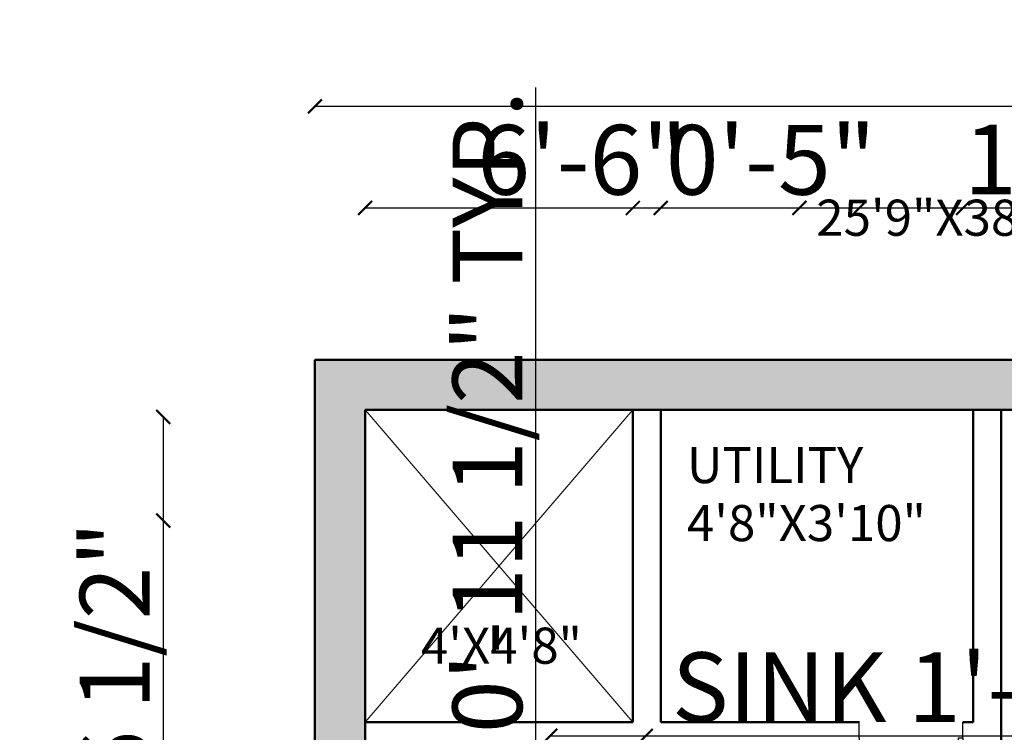
# Model space of a CAD drawing. Units: inches. Extents: x 2419 to 2878, y 1068 to 1713.
# Tile 15 of 20: x 2419 to 2595, y 1511 to 1639. Entities that reach past the tile are written whole.
import ezdxf

# ---------------------------------------------------------------- set-up
doc = ezdxf.new("R2010")
doc.units = ezdxf.units.IN
for name, color, linetype, lineweight in [('A-ANNO-DIMS', 2, 'Continuous', 18), ('A-ANNO-TEXT', 7, 'Continuous', 25), ('A-AREA-IDEN', 7, 'Continuous', 18), ('A-DOOR', 4, 'Continuous', 25), ('A-FLOR-OTLN', 8, 'Continuous', 13), ('A-FLOR-PRKG-PATT', 1, 'Continuous', 13), ('A-FURN-PATT', 254, 'Continuous', 13), ('A-WALL', 7, 'Continuous', 50)]:
    doc.layers.add(name, color=color, linetype=linetype, lineweight=lineweight)
doc.layers.add('A-FLOR-FIXT-PATT', color=254, linetype='Continuous', lineweight=13, true_color=0xd7ebd2)
doc.layers.add('A-WALL-PATT', color=18, linetype='Continuous', lineweight=13, true_color=0x000000)
doc.styles.get("Standard").update_dxf_attribs({"font": 'arial.ttf'})
doc.dimstyles.new('ISO-25', dxfattribs={"dimtxt": 12.5, "dimasz": 2.5, "dimexe": 1.25, "dimexo": 0.625, "dimtad": 1, "dimdec": 0, "dimlunit": 4, "dimtxsty": 'Standard', "dimblk": 'ARCHTICK', "dimcen": 2.5, "dimse1": 1, "dimse2": 1, "dimclrd": 4, "dimadec": 0, "dimazin": 0, "dimtfac": 1, "dimtdec": 0, "dimtmove": 0, "dimatfit": 3, "dimfxl": 1, "dimarcsym": 0})

# ---------------------------------------------------------------- blocks, each defined once
blk = doc.blocks.new('*U3')
for p, q in [((0, 0), (0, -6)), ((40, 0), (40, -6))]:
    blk.add_line(p, q)
blk.add_lwpolyline([(0, 0), (0, 40), (1.75, 40), (1.75, 0)], close=True)
blk.add_arc((0, 0), 40, 0, 90)
blk = doc.blocks.new('_ArchTick')
at = {"color": 0, "linetype": 'ByBlock', "const_width": 0.15}
blk.add_lwpolyline([(-0.5, -0.5), (0.5, 0.5)], dxfattribs=at)
blk = doc.blocks.new('*D16')
at = {"layer": 'A-ANNO-DIMS', "color": 0, "lineweight": -2, "transparency": 16777216}
blk.add_line((2471.51, 1623.24), (2780.51, 1623.24), dxfattribs=at)
at = {"layer": 'Defpoints', "color": 0, "transparency": 16777216}
for p in [(2780.51, 1623.24), (2471.51, 1577.81), (2780.51, 1577.81)]:
    blk.add_point(p, dxfattribs=at)
at = {"layer": 'A-ANNO-DIMS', "color": 0, "lineweight": -2, "transparency": 16777216, "xscale": 2.5, "yscale": 2.5, "zscale": 2.5, "rotation": 180}
blk.add_blockref('_ArchTick', (2471.51, 1623.24), dxfattribs=at)
at = {"layer": 'A-ANNO-DIMS', "color": 0, "lineweight": -2, "transparency": 16777216, "xscale": 2.5, "yscale": 2.5, "zscale": 2.5}
blk.add_blockref('_ArchTick', (2780.51, 1623.24), dxfattribs=at)
at = {"layer": 'A-ANNO-DIMS', "color": 0, "transparency": 16777216, "insert": (2626.01, 1630.25), "char_height": 12.5, "attachment_point": 5}
blk.add_mtext('25\'-9"', dxfattribs=at)
blk = doc.blocks.new('*D22')
at = {"layer": 'A-ANNO-DIMS', "color": 4, "lineweight": -2, "transparency": 16777216}
for p, q in [((2513.7, 1510.38), (2530.82, 1510.38)), ((2530.82, 1510.38), (2656.31, 1510.38))]:
    blk.add_line(p, q, dxfattribs=at)
at = {"layer": 'Defpoints', "color": 0, "transparency": 16777216}
for p in [(2530.82, 1510.38), (2513.7, 1507.81), (2530.82, 1507.81)]:
    blk.add_point(p, dxfattribs=at)
at = {"layer": 'A-ANNO-DIMS', "color": 4, "lineweight": -2, "transparency": 16777216, "xscale": 2.5, "yscale": 2.5, "zscale": 2.5, "rotation": 180}
blk.add_blockref('_ArchTick', (2513.7, 1510.38), dxfattribs=at)
at = {"layer": 'A-ANNO-DIMS', "color": 4, "lineweight": -2, "transparency": 16777216, "xscale": 2.5, "yscale": 2.5, "zscale": 2.5}
blk.add_blockref('_ArchTick', (2530.82, 1510.38), dxfattribs=at)
at = {"layer": 'A-ANNO-DIMS', "color": 0, "transparency": 16777216, "insert": (2594.82, 1517.47), "char_height": 12.5, "attachment_point": 5}
blk.add_mtext('SINK 1\'-5" TYP.', dxfattribs=at)
blk = doc.blocks.new('*D23')
at = {"layer": 'A-ANNO-DIMS', "color": 4, "lineweight": -2, "transparency": 16777216}
for p, q in [((2511.14, 1507.81), (2511.14, 1626.6)), ((2511.14, 1496.4), (2511.14, 1507.81))]:
    blk.add_line(p, q, dxfattribs=at)
at = {"layer": 'Defpoints', "color": 0, "transparency": 16777216}
for p in [(2511.14, 1507.81), (2513.7, 1507.81), (2513.7, 1496.4)]:
    blk.add_point(p, dxfattribs=at)
at = {"layer": 'A-ANNO-DIMS', "color": 4, "lineweight": -2, "transparency": 16777216, "xscale": 2.5, "yscale": 2.5, "zscale": 2.5}
for p, rotation in [((2511.14, 1507.81), 90), ((2511.14, 1496.4), 270)]:
    blk.add_blockref('_ArchTick', p, dxfattribs=dict(at, rotation=rotation))
at = {"layer": 'A-ANNO-DIMS', "color": 0, "transparency": 16777216, "insert": (2504.05, 1568.45), "char_height": 12.5, "attachment_point": 5, "rotation": 90}
blk.add_mtext('0\'-11 1/2" TYP.', dxfattribs=at)
blk = doc.blocks.new('*D42')
at = {"layer": 'A-ANNO-DIMS', "color": 4, "lineweight": -2, "transparency": 16777216}
for p, q in [((2528.51, 1605.01), (2533.51, 1605.01)), ((2533.51, 1605.01), (2570.49, 1605.01))]:
    blk.add_line(p, q, dxfattribs=at)
at = {"layer": 'Defpoints', "color": 0, "transparency": 16777216}
for p in [(2533.51, 1605.01), (2528.51, 1568.81), (2533.51, 1568.81)]:
    blk.add_point(p, dxfattribs=at)
at = {"layer": 'A-ANNO-DIMS', "color": 4, "lineweight": -2, "transparency": 16777216, "xscale": 2.5, "yscale": 2.5, "zscale": 2.5, "rotation": 180}
blk.add_blockref('_ArchTick', (2528.51, 1605.01), dxfattribs=at)
at = {"layer": 'A-ANNO-DIMS', "color": 4, "lineweight": -2, "transparency": 16777216, "xscale": 2.5, "yscale": 2.5, "zscale": 2.5}
blk.add_blockref('_ArchTick', (2533.51, 1605.01), dxfattribs=at)
at = {"layer": 'A-ANNO-DIMS', "color": 0, "transparency": 16777216, "insert": (2553.25, 1612.02), "char_height": 12.5, "attachment_point": 5}
blk.add_mtext('0\'-5"', dxfattribs=at)
blk = doc.blocks.new('*D46')
at = {"layer": 'A-ANNO-DIMS', "color": 4, "lineweight": -2, "transparency": 16777216}
for p, q in [((2569.11, 1605.01), (2587.69, 1605.01)), ((2587.69, 1605.01), (2652.62, 1605.01))]:
    blk.add_line(p, q, dxfattribs=at)
at = {"layer": 'Defpoints', "color": 0, "transparency": 16777216}
for p in [(2587.69, 1605.01), (2569.11, 1512.81), (2587.69, 1512.81)]:
    blk.add_point(p, dxfattribs=at)
at = {"layer": 'A-ANNO-DIMS', "color": 4, "lineweight": -2, "transparency": 16777216, "xscale": 2.5, "yscale": 2.5, "zscale": 2.5, "rotation": 180}
blk.add_blockref('_ArchTick', (2569.11, 1605.01), dxfattribs=at)
at = {"layer": 'A-ANNO-DIMS', "color": 4, "lineweight": -2, "transparency": 16777216, "xscale": 2.5, "yscale": 2.5, "zscale": 2.5}
blk.add_blockref('_ArchTick', (2587.69, 1605.01), dxfattribs=at)
at = {"layer": 'A-ANNO-DIMS', "color": 0, "transparency": 16777216, "insert": (2621.41, 1612.1), "char_height": 12.5, "attachment_point": 5}
blk.add_mtext('1\'-6 1/2"', dxfattribs=at)
blk = doc.blocks.new('*D48')
at = {"layer": 'A-ANNO-DIMS', "color": 4, "lineweight": -2, "transparency": 16777216}
for p, q in [((2444.31, 1567.55), (2444.31, 1548.96)), ((2444.31, 1548.96), (2444.31, 1484.03))]:
    blk.add_line(p, q, dxfattribs=at)
at = {"layer": 'Defpoints', "color": 0, "transparency": 16777216}
for p in [(2725.51, 1567.55), (2444.31, 1548.96), (2725.51, 1548.96)]:
    blk.add_point(p, dxfattribs=at)
at = {"layer": 'A-ANNO-DIMS', "color": 4, "lineweight": -2, "transparency": 16777216, "xscale": 2.5, "yscale": 2.5, "zscale": 2.5}
for p, rotation in [((2444.31, 1567.55), 90), ((2444.31, 1548.96), 270)]:
    blk.add_blockref('_ArchTick', p, dxfattribs=dict(at, rotation=rotation))
at = {"layer": 'A-ANNO-DIMS', "color": 0, "transparency": 16777216, "insert": (2437.23, 1515.25), "char_height": 12.5, "attachment_point": 5, "rotation": 90}
blk.add_mtext('1\'-6 1/2"', dxfattribs=at)
blk = doc.blocks.new('*D57')
at = {"layer": 'A-ANNO-DIMS', "color": 4, "lineweight": -2, "transparency": 16777216}
blk.add_line((2480.51, 1605.01), (2558.38, 1605.01), dxfattribs=at)
at = {"layer": 'Defpoints', "color": 0, "transparency": 16777216}
for p in [(2558.38, 1605.01), (2480.51, 1507.81), (2558.38, 1507.81)]:
    blk.add_point(p, dxfattribs=at)
at = {"layer": 'A-ANNO-DIMS', "color": 4, "lineweight": -2, "transparency": 16777216, "xscale": 2.5, "yscale": 2.5, "zscale": 2.5, "rotation": 180}
blk.add_blockref('_ArchTick', (2480.51, 1605.01), dxfattribs=at)
at = {"layer": 'A-ANNO-DIMS', "color": 4, "lineweight": -2, "transparency": 16777216, "xscale": 2.5, "yscale": 2.5, "zscale": 2.5}
blk.add_blockref('_ArchTick', (2558.38, 1605.01), dxfattribs=at)
at = {"layer": 'A-ANNO-DIMS', "color": 0, "transparency": 16777216, "insert": (2519.45, 1612.02), "char_height": 12.5, "attachment_point": 5}
blk.add_mtext('6\'-6"', dxfattribs=at)

msp = doc.modelspace()

# ---------------------------------------------------------------- hatches: boundary and pattern name
at = {"layer": 'A-FLOR-FIXT-PATT'}
h = msp.add_hatch(color=256, dxfattribs=at)
h.dxf.hatch_style = 1
h.paths.add_polyline_path([(2771.51, 1458.39), (2763.51, 1458.39), (2763.51, 1437.39), (2771.51, 1437.39)])
h.paths.add_polyline_path([(2770.51, 1456.39, 0.5), (2769.51, 1457.39), (2765.51, 1457.39, 0.5), (2764.51, 1456.39), (2764.51, 1439.39, 0.5), (2765.51, 1438.39), (2769.51, 1438.39, 0.5), (2770.51, 1439.39)], flags=16)
h.paths.add_polyline_path([(2706.38, 1408.81), (2685.38, 1408.81), (2685.38, 1400.81), (2706.38, 1400.81)])
h.paths.add_polyline_path([(2704.38, 1401.81, 0.5), (2705.38, 1402.81), (2705.38, 1406.81, 0.5), (2704.38, 1407.81), (2687.38, 1407.81, 0.5), (2686.38, 1406.81), (2686.38, 1402.81, 0.5), (2687.38, 1401.81)], flags=16)
h.paths.add_polyline_path([(2574.48, 1207.45), (2633.94, 1207.45), (2633.94, 1217.37), (2574.48, 1217.37)], flags=9)
h.paths.add_polyline_path([(2574.45, 1217.83), (2610.47, 1217.83), (2610.47, 1227.88), (2574.45, 1227.88)], flags=9)
h.paths.add_polyline_path([(2672.43, 1304.02), (2718.62, 1304.02), (2718.62, 1313.94), (2672.43, 1313.94)], flags=9)
h.paths.add_polyline_path([(2672.4, 1314.4), (2750.13, 1314.4), (2750.13, 1324.45), (2672.4, 1324.45)], flags=9)
h.paths.add_polyline_path([(2500.43, 1374.44), (2544.8, 1374.44), (2544.8, 1384.36), (2500.43, 1384.36)], flags=9)
h.paths.add_polyline_path([(2500.41, 1384.82), (2566.08, 1384.82), (2566.08, 1394.87), (2500.41, 1394.87)], flags=9)
h.paths.add_polyline_path([(2738.93, 1376.75), (2778.27, 1376.75), (2778.27, 1386.67), (2738.93, 1386.67)], flags=9)
h.paths.add_polyline_path([(2659.12, 1357.8), (2703.49, 1357.8), (2703.49, 1367.72), (2659.12, 1367.72)], flags=9)
h.paths.add_polyline_path([(2659.1, 1368.18), (2694.11, 1368.18), (2694.11, 1378.23), (2659.1, 1378.23)], flags=9)
h.paths.add_polyline_path([(2730.12, 1466.07), (2769.46, 1466.07), (2769.46, 1475.99), (2730.12, 1475.99)], flags=9)
h.paths.add_polyline_path([(2730.1, 1476.45), (2765.12, 1476.45), (2765.12, 1486.5), (2730.1, 1486.5)], flags=9)
h.paths.add_polyline_path([(2730.38, 1518.65), (2761.48, 1518.65), (2761.48, 1528.57), (2730.38, 1528.57)], flags=9)
h.paths.add_polyline_path([(2730.36, 1529.03), (2780.96, 1529.03), (2780.96, 1539.07), (2730.36, 1539.07)], flags=9)
h.paths.add_polyline_path([(2629.32, 1455.19), (2688.78, 1455.19), (2688.78, 1465.11), (2629.32, 1465.11)], flags=9)
h.paths.add_polyline_path([(2629.3, 1465.57), (2681.9, 1465.57), (2681.9, 1475.62), (2629.3, 1475.62)], flags=9)
h.paths.add_polyline_path([(2513.23, 1456.48), (2562.63, 1456.48), (2562.63, 1466.4), (2513.23, 1466.4)], flags=9)
h.paths.add_polyline_path([(2513.21, 1466.86), (2556.26, 1466.86), (2556.26, 1476.91), (2513.21, 1476.91)], flags=9)
h.paths.add_polyline_path([(2488.87, 1521.54), (2519.97, 1521.54), (2519.97, 1531.46), (2488.87, 1531.46)], flags=9)
h.paths.add_polyline_path([(2536.55, 1543.51), (2580.92, 1543.51), (2580.92, 1553.43), (2536.55, 1553.43)], flags=9)
h.paths.add_polyline_path([(2536.56, 1553.92), (2573.53, 1553.92), (2573.53, 1563.8), (2536.56, 1563.8)], flags=9)
at = {"layer": 'A-FLOR-PRKG-PATT'}
h = msp.add_hatch(color=256, dxfattribs=at)
h.dxf.hatch_style = 1
edge = h.paths.add_edge_path()
edge.add_ellipse((2561.37, 1279.45), major_axis=(3.99, 0), ratio=0.842304, start_angle=0.6466, end_angle=90)
edge.add_line((2561.37, 1282.81), (2511.57, 1282.81))
edge.add_ellipse((2511.57, 1279.45), major_axis=(3.99, 0), ratio=0.842304, start_angle=90, end_angle=179.3534)
edge.add_ellipse((10560.89, 1188.62), major_axis=(-8054.03, 0), ratio=0.8423039, start_angle=-0.646554, end_angle=-0.628237)
edge.add_ellipse((2509.23, 1276.91), major_axis=(1.69, 0), ratio=0.842304, start_angle=179.3718, end_angle=248.4648)
edge.add_ellipse((10560.33, 1188.62), major_axis=(8052.29, 0), ratio=0.8423039, start_angle=179.353446, end_angle=179.381357, ccw=False)
edge.add_ellipse((2511.01, 1279.45), major_axis=(2.25, 0), ratio=0.842304, start_angle=90, end_angle=179.3534, ccw=False)
edge.add_line((2511.01, 1281.35), (2561.94, 1281.35))
edge.add_ellipse((2561.94, 1279.45), major_axis=(-2.25, 0), ratio=0.842304, start_angle=180.6466, end_angle=270, ccw=False)
edge.add_ellipse((-5487.38, 1188.62), major_axis=(8052.29, 0), ratio=0.8423039, start_angle=0.528271, end_angle=0.646554, ccw=False)
edge.add_ellipse((2563.71, 1276.91), major_axis=(-1.69, 0), ratio=0.842304, start_angle=111.5352, end_angle=180.6282)
edge.add_ellipse((-5487.95, 1188.62), major_axis=(-8054.03, 0), ratio=0.8423039, start_angle=180.628237, end_angle=180.646554)
edge = h.paths.add_edge_path()
edge.add_ellipse((2564.91, 1261.91), major_axis=(-1.12, 0), ratio=0.842304, start_angle=180, end_angle=270)
edge.add_line((2564.91, 1262.86), (2564.43, 1262.86))
edge.add_ellipse((-5487.38, 1188.62), major_axis=(8052.29, 0), ratio=0.8423039, start_angle=0.383867, end_angle=0.528271, ccw=False)
edge.add_line((2564.65, 1242.56), (2564.91, 1242.56))
edge.add_ellipse((2564.91, 1243.51), major_axis=(-1.12, 0), ratio=0.842304, start_angle=90, end_angle=180)
edge.add_line((2566.03, 1243.51), (2566.03, 1261.91))
edge = h.paths.add_edge_path()
edge.add_ellipse((2564.91, 1174.99), major_axis=(1.12, 0), ratio=0.842304, start_angle=0, end_angle=90)
edge.add_line((2564.91, 1175.94), (2564.89, 1175.94))
edge.add_ellipse((-5487.38, 1188.62), major_axis=(8052.29, 0), ratio=0.8423039, start_angle=-0.134987, end_angle=-0.090229, ccw=False)
edge.add_ellipse((2163.34, 1170.91), major_axis=(401.54, 0), ratio=0.842304, start_angle=-2.18, end_angle=-0.1356, ccw=False)
edge.add_line((2564.47, 1155.64), (2564.91, 1155.64))
edge.add_ellipse((2564.91, 1156.59), major_axis=(-1.12, 0), ratio=0.842304, start_angle=90, end_angle=180)
edge.add_line((2566.03, 1156.59), (2566.03, 1174.99))
h.paths.add_polyline_path([(2574.48, 1207.45), (2633.94, 1207.45), (2633.94, 1217.37), (2574.48, 1217.37)], flags=9)
h.paths.add_polyline_path([(2574.45, 1217.83), (2610.47, 1217.83), (2610.47, 1227.88), (2574.45, 1227.88)], flags=9)
h.paths.add_polyline_path([(2672.43, 1304.02), (2718.62, 1304.02), (2718.62, 1313.94), (2672.43, 1313.94)], flags=9)
h.paths.add_polyline_path([(2672.4, 1314.4), (2750.13, 1314.4), (2750.13, 1324.45), (2672.4, 1324.45)], flags=9)
h.paths.add_polyline_path([(2500.43, 1374.44), (2544.8, 1374.44), (2544.8, 1384.36), (2500.43, 1384.36)], flags=9)
h.paths.add_polyline_path([(2500.41, 1384.82), (2566.08, 1384.82), (2566.08, 1394.87), (2500.41, 1394.87)], flags=9)
h.paths.add_polyline_path([(2738.93, 1376.75), (2778.27, 1376.75), (2778.27, 1386.67), (2738.93, 1386.67)], flags=9)
h.paths.add_polyline_path([(2659.12, 1357.8), (2703.49, 1357.8), (2703.49, 1367.72), (2659.12, 1367.72)], flags=9)
h.paths.add_polyline_path([(2659.1, 1368.18), (2694.11, 1368.18), (2694.11, 1378.23), (2659.1, 1378.23)], flags=9)
h.paths.add_polyline_path([(2730.12, 1466.07), (2769.46, 1466.07), (2769.46, 1475.99), (2730.12, 1475.99)], flags=9)
h.paths.add_polyline_path([(2730.1, 1476.45), (2765.12, 1476.45), (2765.12, 1486.5), (2730.1, 1486.5)], flags=9)
h.paths.add_polyline_path([(2730.38, 1518.65), (2761.48, 1518.65), (2761.48, 1528.57), (2730.38, 1528.57)], flags=9)
h.paths.add_polyline_path([(2730.36, 1529.03), (2780.96, 1529.03), (2780.96, 1539.07), (2730.36, 1539.07)], flags=9)
h.paths.add_polyline_path([(2629.32, 1455.19), (2688.78, 1455.19), (2688.78, 1465.11), (2629.32, 1465.11)], flags=9)
h.paths.add_polyline_path([(2629.3, 1465.57), (2681.9, 1465.57), (2681.9, 1475.62), (2629.3, 1475.62)], flags=9)
h.paths.add_polyline_path([(2513.23, 1456.48), (2562.63, 1456.48), (2562.63, 1466.4), (2513.23, 1466.4)], flags=9)
h.paths.add_polyline_path([(2513.21, 1466.86), (2556.26, 1466.86), (2556.26, 1476.91), (2513.21, 1476.91)], flags=9)
h.paths.add_polyline_path([(2488.87, 1521.54), (2519.97, 1521.54), (2519.97, 1531.46), (2488.87, 1531.46)], flags=9)
h.paths.add_polyline_path([(2536.55, 1543.51), (2580.92, 1543.51), (2580.92, 1553.43), (2536.55, 1553.43)], flags=9)
h.paths.add_polyline_path([(2536.56, 1553.92), (2573.53, 1553.92), (2573.53, 1563.8), (2536.56, 1563.8)], flags=9)
at = {"layer": 'A-FURN-PATT'}
h = msp.add_hatch(color=256, dxfattribs=at)
h.dxf.hatch_style = 1
h.paths.add_polyline_path([(2710.17, 1562.64), (2707.17, 1559.64), (2709.17, 1559.64, -0.414214), (2710.17, 1560.64)])
h.paths.add_polyline_path([(2711.17, 1559.64, 1), (2709.17, 1559.64, 1)])
h.paths.add_polyline_path([(2710.17, 1562.64), (2710.17, 1560.64, -0.414214), (2711.17, 1559.64), (2713.17, 1559.64)])
h.paths.add_polyline_path([(2713.17, 1559.64), (2711.17, 1559.64, -0.414214), (2710.17, 1558.64), (2710.17, 1556.64)])
h.paths.add_polyline_path([(2710.17, 1558.64, -0.414214), (2709.17, 1559.64), (2707.17, 1559.64), (2710.17, 1556.64)])
h.paths.add_polyline_path([(2613.13, 1558.89, 1), (2611.13, 1558.89, 1)])
h.paths.add_polyline_path([(2612.13, 1561.89), (2612.13, 1559.89, -0.414214), (2613.13, 1558.89), (2615.13, 1558.89)])
h.paths.add_polyline_path([(2612.13, 1559.89), (2612.13, 1561.89), (2609.13, 1558.89), (2611.13, 1558.89, -0.414214)])
h.paths.add_polyline_path([(2612.13, 1557.89, -0.414214), (2611.13, 1558.89), (2609.13, 1558.89), (2612.13, 1555.89)])
h.paths.add_polyline_path([(2574.48, 1207.45), (2633.94, 1207.45), (2633.94, 1217.37), (2574.48, 1217.37)], flags=9)
h.paths.add_polyline_path([(2574.45, 1217.83), (2610.47, 1217.83), (2610.47, 1227.88), (2574.45, 1227.88)], flags=9)
h.paths.add_polyline_path([(2672.43, 1304.02), (2718.62, 1304.02), (2718.62, 1313.94), (2672.43, 1313.94)], flags=9)
h.paths.add_polyline_path([(2672.4, 1314.4), (2750.13, 1314.4), (2750.13, 1324.45), (2672.4, 1324.45)], flags=9)
h.paths.add_polyline_path([(2500.43, 1374.44), (2544.8, 1374.44), (2544.8, 1384.36), (2500.43, 1384.36)], flags=9)
h.paths.add_polyline_path([(2500.41, 1384.82), (2566.08, 1384.82), (2566.08, 1394.87), (2500.41, 1394.87)], flags=9)
h.paths.add_polyline_path([(2738.93, 1376.75), (2778.27, 1376.75), (2778.27, 1386.67), (2738.93, 1386.67)], flags=9)
h.paths.add_polyline_path([(2659.12, 1357.8), (2703.49, 1357.8), (2703.49, 1367.72), (2659.12, 1367.72)], flags=9)
h.paths.add_polyline_path([(2659.1, 1368.18), (2694.11, 1368.18), (2694.11, 1378.23), (2659.1, 1378.23)], flags=9)
h.paths.add_polyline_path([(2730.12, 1466.07), (2769.46, 1466.07), (2769.46, 1475.99), (2730.12, 1475.99)], flags=9)
h.paths.add_polyline_path([(2730.1, 1476.45), (2765.12, 1476.45), (2765.12, 1486.5), (2730.1, 1486.5)], flags=9)
h.paths.add_polyline_path([(2730.38, 1518.65), (2761.48, 1518.65), (2761.48, 1528.57), (2730.38, 1528.57)], flags=9)
h.paths.add_polyline_path([(2730.36, 1529.03), (2780.96, 1529.03), (2780.96, 1539.07), (2730.36, 1539.07)], flags=9)
h.paths.add_polyline_path([(2629.32, 1455.19), (2688.78, 1455.19), (2688.78, 1465.11), (2629.32, 1465.11)], flags=9)
h.paths.add_polyline_path([(2629.3, 1465.57), (2681.9, 1465.57), (2681.9, 1475.62), (2629.3, 1475.62)], flags=9)
h.paths.add_polyline_path([(2513.23, 1456.48), (2562.63, 1456.48), (2562.63, 1466.4), (2513.23, 1466.4)], flags=9)
h.paths.add_polyline_path([(2513.21, 1466.86), (2556.26, 1466.86), (2556.26, 1476.91), (2513.21, 1476.91)], flags=9)
h.paths.add_polyline_path([(2488.87, 1521.54), (2519.97, 1521.54), (2519.97, 1531.46), (2488.87, 1531.46)], flags=9)
h.paths.add_polyline_path([(2536.55, 1543.51), (2580.92, 1543.51), (2580.92, 1553.43), (2536.55, 1553.43)], flags=9)
h.paths.add_polyline_path([(2536.56, 1553.92), (2573.53, 1553.92), (2573.53, 1563.8), (2536.56, 1563.8)], flags=9)
at = {"layer": 'A-WALL-PATT'}
h = msp.add_hatch(color=256, dxfattribs=at)
h.dxf.hatch_style = 1
h.paths.add_polyline_path([(2780.51, 1577.81), (2471.51, 1577.81), (2471.51, 1121.81), (2780.51, 1121.81)])
h.paths.add_polyline_path([(2480.51, 1568.81), (2771.51, 1568.81), (2771.51, 1130.81), (2480.51, 1130.81)], flags=16)
h.paths.add_polyline_path([(2528.51, 1568.81), (2528.51, 1512.81), (2594.51, 1512.81), (2594.51, 1414.81), (2596.57, 1414.81), (2596.57, 1441.61), (2597.82, 1441.61), (2597.82, 1441.58, -0.384016), (2625.03, 1414.81), (2725.51, 1414.81), (2725.51, 1567.55), (2728.3, 1567.55), (2746.89, 1567.55), (2746.89, 1566.73), (2746.87, 1566.73, -0.367216), (2730.51, 1549.09), (2730.51, 1512.81), (2750.85, 1512.81), (2750.85, 1510.03, -0.401453), (2733.08, 1491.46), (2733.08, 1491.44), (2732.27, 1491.44), (2732.27, 1507.81), (2730.51, 1507.81), (2730.51, 1408.81), (2736.51, 1408.81), (2736.51, 1349.81), (2632.51, 1349.81), (2632.51, 1408.81), (2528.51, 1408.81), (2528.51, 1414.81), (2503.97, 1414.81), (2503.97, 1494.85), (2558.38, 1494.85), (2558.38, 1507.81), (2529.96, 1507.81, -0.414214), (2530.82, 1506.96), (2530.82, 1497.26, -0.414214), (2529.96, 1496.4), (2514.56, 1496.4, -0.414214), (2513.7, 1497.26), (2513.7, 1506.96, -0.414214), (2514.56, 1507.81), (2528.51, 1507.81), (2528.51, 1512.81), (2480.51, 1512.81)], flags=0)
h.paths.add_polyline_path([(2516.26, 1507.81), (2528.26, 1507.81), (2528.26, 1505.81), (2523.42, 1505.81), (2524.07, 1504.67), (2529.39, 1504.67, -0.414214), (2529.96, 1504.1), (2529.96, 1497.83, -0.414214), (2529.39, 1497.26), (2515.13, 1497.26, -0.414214), (2514.56, 1497.83), (2514.56, 1504.1, -0.414214), (2515.13, 1504.67), (2520.69, 1504.67), (2521.34, 1505.81), (2516.26, 1505.81)], flags=0)
h.paths.add_polyline_path([(2522.02, 1505.53), (2522.82, 1507.32, -0.65506), (2522.25, 1506.06), (2522.19, 1505.93), (2522.43, 1505.53)], flags=0)
h.paths.add_polyline_path([(2522.83, 1500.97, -1), (2521.69, 1500.97, -1)], flags=0)
h.paths.add_polyline_path([(2522.55, 1500.97, -1), (2521.98, 1500.97, -1)], flags=0)
h.paths.add_polyline_path([(2482.01, 1470.63), (2499.89, 1470.63), (2499.89, 1448.27), (2482.01, 1448.27), (2482.01, 1452.74), (2481.26, 1452.74), (2481.26, 1449.76), (2480.51, 1449.76), (2480.51, 1469.14), (2481.26, 1469.14), (2481.26, 1466.16), (2482.01, 1466.16)], flags=0)
h.paths.add_polyline_path([(2488.71, 1466.16, -1), (2484.24, 1466.16, -1)], flags=0)
h.paths.add_polyline_path([(2496.17, 1466.16, -1), (2490.2, 1466.16, -1)], flags=0)
h.paths.add_polyline_path([(2487.97, 1466.16, -1), (2484.99, 1466.16, -1)], flags=0)
h.paths.add_polyline_path([(2495.42, 1466.16, -1), (2490.95, 1466.16, -1)], flags=0)
h.paths.add_polyline_path([(2487.22, 1466.16, -1), (2485.73, 1466.16, -1)], flags=0)
h.paths.add_polyline_path([(2494.68, 1466.16, -1), (2491.69, 1466.16, -1)], flags=0)
h.paths.add_polyline_path([(2499.11, 1468, -1), (2497.98, 1468, -1)], flags=0)
h.paths.add_polyline_path([(2493.93, 1466.16, -1), (2492.44, 1466.16, -1)], flags=0)
h.paths.add_polyline_path([(2499.37, 1463.71, -1), (2498.17, 1463.71, -1)], flags=0)
h.paths.add_polyline_path([(2484.24, 1461.69), (2496.17, 1461.69), (2496.17, 1457.22), (2484.24, 1457.22)], flags=0)
h.paths.add_polyline_path([(2484.99, 1460.94), (2495.42, 1460.94), (2495.42, 1457.96), (2484.99, 1457.96)], flags=0)
h.paths.add_polyline_path([(2586.88, 1510.03), (2587.69, 1510.03), (2587.69, 1491.44), (2586.88, 1491.44)], flags=0)
h.paths.add_polyline_path([(2499.26, 1459.41, -1), (2498.2, 1459.41, -1)], flags=0)
h.paths.add_polyline_path([(2489.46, 1452.74, -1), (2483.5, 1452.74, -1)], flags=0)
h.paths.add_polyline_path([(2557.3, 1408.81), (2557.3, 1413.09, -0.401453), (2584.57, 1441.58), (2584.57, 1441.61), (2585.82, 1441.61), (2585.82, 1413.09), (2585.82, 1408.81)], flags=0)
h.paths.add_polyline_path([(2488.71, 1452.74, -1), (2484.24, 1452.74, -1)], flags=0)
h.paths.add_polyline_path([(2495.42, 1452.74, -1), (2490.95, 1452.74, -1)], flags=0)
h.paths.add_polyline_path([(2487.97, 1452.74, -1), (2484.99, 1452.74, -1)], flags=0)
h.paths.add_polyline_path([(2494.68, 1452.74, -1), (2491.69, 1452.74, -1)], flags=0)
h.paths.add_polyline_path([(2487.22, 1452.74, -1), (2485.73, 1452.74, -1)], flags=0)
h.paths.add_polyline_path([(2499.18, 1454.44, -1), (2497.9, 1454.44, -1)], flags=0)
h.paths.add_polyline_path([(2493.93, 1452.74, -1), (2492.44, 1452.74, -1)], flags=0)
h.paths.add_polyline_path([(2499.3, 1450.64, -1), (2497.79, 1450.64, -1)], flags=0)
h.paths.add_polyline_path([(2619.13, 1558.89, -1), (2605.13, 1558.89, -1)], flags=0)
h.paths.add_polyline_path([(2609.13, 1558.89), (2612.13, 1561.89), (2615.13, 1558.89), (2612.13, 1555.89)], flags=0)
h.paths.add_polyline_path([(2611.13, 1558.89, -1), (2613.13, 1558.89, -1)], flags=0)
h.paths.add_polyline_path([(2633.68, 1568.81), (2693.68, 1568.81), (2693.68, 1488.81), (2633.68, 1488.81)], flags=0)
h.paths.add_polyline_path([(2641.68, 1554.41), (2641.68, 1567.61), (2662.48, 1567.61), (2662.48, 1554.41), (2664.88, 1554.41), (2664.88, 1567.61), (2685.68, 1567.61), (2685.68, 1552.41), (2680.48, 1552.41), (2693.68, 1539.21), (2678.48, 1539.21), (2678.48, 1554.41)], flags=0)
h.paths.add_polyline_path([(2637.51, 1408.81), (2731.51, 1408.81), (2731.51, 1354.81), (2637.51, 1354.81), (2637.51, 1357.98), (2635.3, 1357.98), (2635.3, 1358.79), (2637.51, 1358.79)], flags=0)
h.paths.add_polyline_path([(2717.17, 1559.64, -1), (2703.17, 1559.64, -1)], flags=0)
h.paths.add_polyline_path([(2707.17, 1559.64), (2710.17, 1562.64), (2713.17, 1559.64), (2710.17, 1556.64)], flags=0)
h.paths.add_polyline_path([(2709.17, 1559.64, -1), (2711.17, 1559.64, -1)], flags=0)
h.paths.add_polyline_path([(2685.38, 1408.81), (2706.38, 1408.81), (2706.38, 1400.81), (2699.88, 1400.81), (2701.88, 1394.81, -0.501323), (2696.92, 1375.95, -0.132891), (2694.83, 1375.95, -0.501317), (2689.88, 1394.81), (2691.88, 1400.81), (2688.88, 1400.81), (2688.88, 1399.31), (2685.88, 1399.31), (2685.88, 1400.31), (2687.88, 1400.31), (2687.88, 1400.81), (2685.38, 1400.81)], flags=0)
h.paths.add_polyline_path([(2687.38, 1407.81), (2704.38, 1407.81, -0.5), (2705.38, 1406.81), (2705.38, 1402.81, -0.5), (2704.38, 1401.81), (2687.38, 1401.81, -0.5), (2686.38, 1402.81), (2686.38, 1406.81, -0.5)], flags=0)
h.paths.add_polyline_path([(2639.51, 1205.81), (2634.51, 1205.81), (2634.51, 1293.81), (2637.51, 1293.81), (2639.51, 1293.81)], flags=0)
h.paths.add_polyline_path([(2691.88, 1394.81), (2699.88, 1394.81, -0.48008), (2697.52, 1377.29, -0.215004), (2694.23, 1377.29, -0.48008)], flags=0)
h.paths.add_polyline_path([(2757.51, 1453.89), (2763.51, 1451.89), (2763.51, 1454.89), (2762.01, 1454.89), (2762.01, 1457.89), (2763.01, 1457.89), (2763.01, 1455.89), (2763.51, 1455.89), (2763.51, 1458.39), (2771.51, 1458.39), (2771.51, 1437.39), (2763.51, 1437.39), (2763.51, 1443.89), (2757.51, 1441.89, -0.501323), (2738.65, 1446.85, -0.132891), (2738.65, 1448.94, -0.501317)], flags=0)
h.paths.add_polyline_path([(2739.99, 1449.54, -0.48008), (2757.51, 1451.89), (2757.51, 1443.89, -0.48008), (2739.99, 1446.25, -0.215004)], flags=0)
h.paths.add_polyline_path([(2765.51, 1457.39), (2769.51, 1457.39, -0.5), (2770.51, 1456.39), (2770.51, 1439.39, -0.5), (2769.51, 1438.39), (2765.51, 1438.39, -0.5), (2764.51, 1439.39), (2764.51, 1456.39, -0.5)], flags=0)
h = msp.add_hatch(color=256, dxfattribs=at)
h.dxf.hatch_style = 1
h.paths.add_polyline_path([(2771.51, 1354.81), (2736.51, 1354.81), (2736.51, 1408.81), (2771.51, 1408.81), (2771.51, 1414.81), (2625.03, 1414.81, -0.015108), (2625.09, 1413.09), (2625.09, 1408.81), (2632.51, 1408.81), (2632.51, 1376.56), (2635.3, 1376.56, -0.029838), (2637.51, 1376.43), (2637.51, 1408.81), (2731.51, 1408.81), (2731.51, 1354.81), (2637.51, 1354.81), (2637.51, 1357.98), (2635.3, 1357.98), (2632.51, 1357.98), (2632.51, 1349.81), (2771.51, 1349.81)])
h.paths.add_polyline_path([(2639.51, 1298.81), (2637.51, 1298.81), (2480.51, 1298.81), (2480.51, 1293.81), (2637.51, 1293.81), (2639.51, 1293.81)])
h.paths.add_polyline_path([(2639.51, 1293.81), (2637.51, 1293.81), (2634.51, 1293.81), (2634.51, 1244.65), (2638.79, 1244.65, -0.006332), (2639.51, 1244.64)])
h.paths.add_polyline_path([(2639.51, 1205.81), (2771.51, 1205.81), (2771.51, 1210.81), (2639.51, 1210.81), (2639.51, 1216.13), (2638.79, 1216.13), (2634.51, 1216.13), (2634.51, 1130.81), (2639.51, 1130.81)])
h.paths.add_polyline_path([(2596.57, 1413.09), (2596.57, 1414.81), (2585.82, 1414.81), (2585.82, 1413.09), (2585.82, 1408.81), (2596.57, 1408.81)])
h.paths.add_polyline_path([(2557.3, 1413.09, -0.015108), (2557.35, 1414.81), (2480.51, 1414.81), (2480.51, 1408.81), (2557.3, 1408.81)])
h.paths.add_polyline_path([(2574.48, 1207.45), (2633.94, 1207.45), (2633.94, 1217.37), (2574.48, 1217.37)], flags=9)
h.paths.add_polyline_path([(2574.45, 1217.83), (2610.47, 1217.83), (2610.47, 1227.88), (2574.45, 1227.88)], flags=9)
h.paths.add_polyline_path([(2672.43, 1304.02), (2718.62, 1304.02), (2718.62, 1313.94), (2672.43, 1313.94)], flags=9)
h.paths.add_polyline_path([(2672.4, 1314.4), (2750.13, 1314.4), (2750.13, 1324.45), (2672.4, 1324.45)], flags=9)
h.paths.add_polyline_path([(2500.43, 1374.44), (2544.8, 1374.44), (2544.8, 1384.36), (2500.43, 1384.36)], flags=9)
h.paths.add_polyline_path([(2500.41, 1384.82), (2566.08, 1384.82), (2566.08, 1394.87), (2500.41, 1394.87)], flags=9)
h.paths.add_polyline_path([(2738.93, 1376.75), (2778.27, 1376.75), (2778.27, 1386.67), (2738.93, 1386.67)], flags=9)
h.paths.add_polyline_path([(2659.12, 1357.8), (2703.49, 1357.8), (2703.49, 1367.72), (2659.12, 1367.72)], flags=25)
h.paths.add_polyline_path([(2659.1, 1368.18), (2694.11, 1368.18), (2694.11, 1378.23), (2659.1, 1378.23)], flags=25)
h.paths.add_polyline_path([(2730.12, 1466.07), (2769.46, 1466.07), (2769.46, 1475.99), (2730.12, 1475.99)], flags=9)
h.paths.add_polyline_path([(2730.1, 1476.45), (2765.12, 1476.45), (2765.12, 1486.5), (2730.1, 1486.5)], flags=9)
h.paths.add_polyline_path([(2730.38, 1518.65), (2761.48, 1518.65), (2761.48, 1528.57), (2730.38, 1528.57)], flags=9)
h.paths.add_polyline_path([(2730.36, 1529.03), (2780.96, 1529.03), (2780.96, 1539.07), (2730.36, 1539.07)], flags=9)
h.paths.add_polyline_path([(2629.32, 1455.19), (2688.78, 1455.19), (2688.78, 1465.11), (2629.32, 1465.11)], flags=9)
h.paths.add_polyline_path([(2629.3, 1465.57), (2681.9, 1465.57), (2681.9, 1475.62), (2629.3, 1475.62)], flags=9)
h.paths.add_polyline_path([(2513.23, 1456.48), (2562.63, 1456.48), (2562.63, 1466.4), (2513.23, 1466.4)], flags=9)
h.paths.add_polyline_path([(2513.21, 1466.86), (2556.26, 1466.86), (2556.26, 1476.91), (2513.21, 1476.91)], flags=9)
h.paths.add_polyline_path([(2488.87, 1521.54), (2519.97, 1521.54), (2519.97, 1531.46), (2488.87, 1531.46)], flags=9)
h.paths.add_polyline_path([(2536.55, 1543.51), (2580.92, 1543.51), (2580.92, 1553.43), (2536.55, 1553.43)], flags=9)
h.paths.add_polyline_path([(2536.56, 1553.92), (2573.53, 1553.92), (2573.53, 1563.8), (2536.56, 1563.8)], flags=9)

# ---------------------------------------------------------------- linework, layer by layer
at = {"layer": 'A-FLOR-OTLN'}
for p, q in [((2528.51, 1568.81), (2480.51, 1512.81)), ((2480.51, 1568.81), (2528.51, 1512.81))]:
    msp.add_line(p, q, dxfattribs=at)
at = {"layer": 'A-WALL'}
for p, q in [((2480.51, 1568.81), (2771.51, 1568.81)), ((2480.51, 1130.81), (2480.51, 1568.81)), ((2528.51, 1512.81), (2528.51, 1568.81)), ((2533.51, 1512.81), (2533.51, 1568.81)), ((2589.51, 1512.81), (2589.51, 1568.81)), ((2594.51, 1414.81), (2594.51, 1568.81)), ((2480.51, 1512.81), (2528.51, 1512.81)), ((2533.51, 1512.81), (2569.11, 1512.81)), ((2587.69, 1512.81), (2589.51, 1512.81))]:
    msp.add_line(p, q, dxfattribs=at)
msp.add_lwpolyline([(2471.51, 1577.81), (2780.51, 1577.81), (2780.51, 1121.81), (2471.51, 1121.81)], close=True, dxfattribs=at)

# ---------------------------------------------------------------- block references
at = {"layer": 'A-DOOR', "xscale": 0.4646269055216028, "yscale": 0.4646269055216028, "zscale": 0.4646269055216028, "rotation": 180}
msp.add_blockref('*U3', (2587.69, 1510.03), dxfattribs=at)

# ---------------------------------------------------------------- texts
at = {"layer": 'A-ANNO-TEXT'}
msp.add_text('25\'9"X38\' HOUSE PLAN', height=6.4753, dxfattribs=at).set_placement((2561.39, 1600.03))
at = {"layer": 'A-AREA-IDEN'}
for s, p in [('UTILITY', (2538.2, 1555.68)), ('4\'8"X3\'10"', (2538.2, 1545.28)), ('4\'X4\'8"', (2490.52, 1523.3))]:
    msp.add_text(s, height=6.475, dxfattribs=at).set_placement(p)

# ---------------------------------------------------------------- dimensions: what is measured, and where the dimension line sits
at = {"layer": 'A-ANNO-DIMS'}
for base, p1, p2, override, picture, middle in [((2780.51, 1623.24), (2471.51, 1577.81), (2780.51, 1577.81), {"dimclrd": 0, "dimclre": 0, "dimclrt": 0}, '*D16', (2626.01, 1630.25)), ((2587.69, 1605.01), (2569.11, 1512.81), (2587.69, 1512.81), {"dimdec": 1, "dimlfac": 1, "dimrnd": 0, "dimzin": 1, "dimdsep": 46, "dimlunit": 4, "dimfrac": 2}, '*D46', (2621.41, 1612.1)), ((2558.38, 1605.01), (2480.51, 1507.81), (2558.38, 1507.81), {"dimdec": 1, "dimlfac": 1, "dimrnd": 0, "dimzin": 1, "dimdsep": 46, "dimlunit": 4, "dimfrac": 2}, '*D57', (2519.45, 1612.02)), ((2533.51, 1605.01), (2528.51, 1568.81), (2533.51, 1568.81), {"dimdec": 1, "dimlfac": 1, "dimrnd": 0, "dimzin": 1, "dimdsep": 46, "dimlunit": 4, "dimfrac": 2}, '*D42', (2553.25, 1612.02))]:
    dim = msp.add_linear_dim(base=base, p1=p1, p2=p2, dimstyle='ISO-25', override=override, dxfattribs=at)
    dim.commit()
    dim.dimension.update_dxf_attribs({"geometry": picture, "text_midpoint": middle})
dim = msp.add_linear_dim(base=(2511.14, 1507.81), p1=(2513.7, 1496.4), p2=(2513.7, 1507.81), angle=90, text='<> TYP.', dimstyle='ISO-25', override={"dimdec": 1, "dimlfac": 1, "dimrnd": 0, "dimzin": 1, "dimdsep": 46, "dimlunit": 4, "dimfrac": 2}, dxfattribs=at)
dim.commit()
dim.dimension.update_dxf_attribs({"geometry": '*D23', "text_midpoint": (2504.05, 1568.45)})
dim = msp.add_linear_dim(base=(2444.31, 1548.96), p1=(2725.51, 1567.55), p2=(2725.51, 1548.96), angle=90, dimstyle='ISO-25', override={"dimdec": 1, "dimlfac": 1, "dimrnd": 0, "dimzin": 1, "dimdsep": 46, "dimlunit": 4, "dimfrac": 2}, dxfattribs=at)
dim.commit()
dim.dimension.update_dxf_attribs({"geometry": '*D48', "text_midpoint": (2437.23, 1515.25)})
dim = msp.add_linear_dim(base=(2530.82, 1510.38), p1=(2513.7, 1507.81), p2=(2530.82, 1507.81), text='SINK <> TYP.', dimstyle='ISO-25', override={"dimdec": 1, "dimlfac": 1, "dimrnd": 0, "dimzin": 1, "dimdsep": 46, "dimlunit": 4, "dimfrac": 2}, dxfattribs=at)
dim.commit()
dim.dimension.update_dxf_attribs({"geometry": '*D22', "text_midpoint": (2594.82, 1517.47)})

doc.saveas('drawing.dxf')
